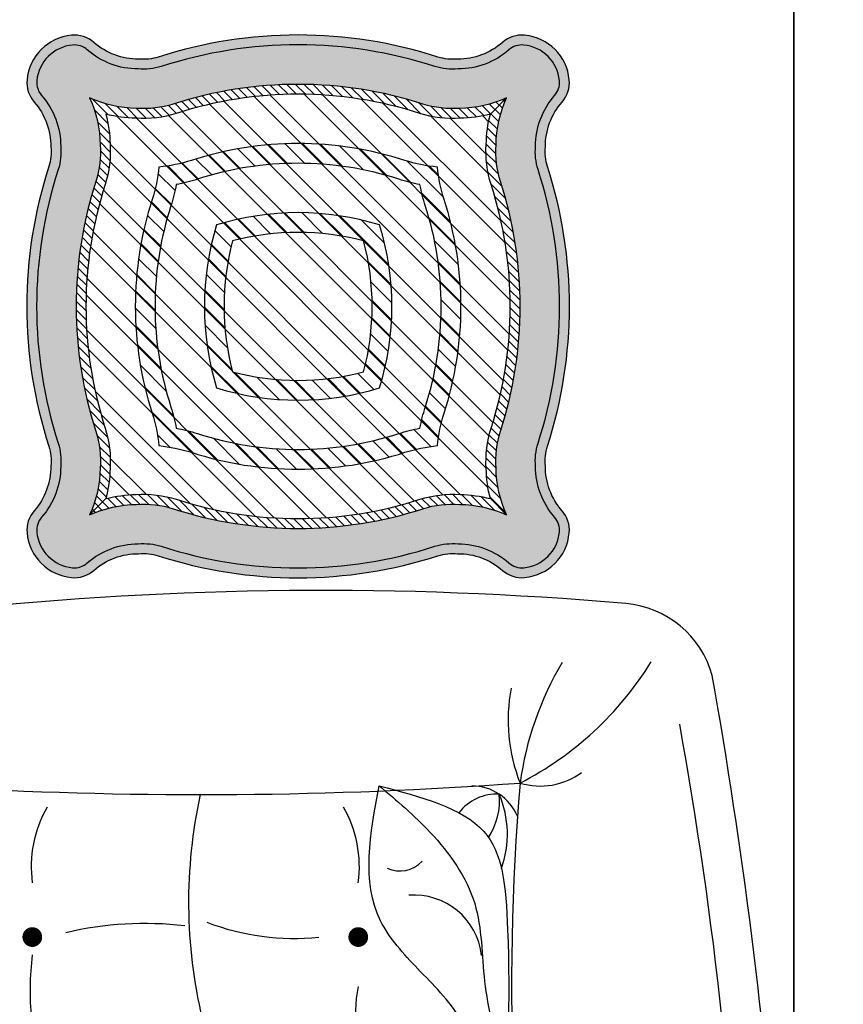
# Model space of a CAD drawing. Units: inches. Extents: x 844 to 2234, y 346 to 1084.
# Tile 88 of 93: x 2017.59 to 2030.9, y 712.93 to 728.83. Entities that reach past the tile are written whole.
import ezdxf

# ---------------------------------------------------------------- set-up
doc = ezdxf.new("R2010")
doc.units = ezdxf.units.IN
doc.header["$MEASUREMENT"] = 0
for name, color, linetype, lineweight in [('A-ANNO-DIMS', 2, 'Continuous', 18), ('A-WALL', 7, 'Continuous', 35), ('furniture', 8, 'Continuous', 18)]:
    doc.layers.add(name, color=color, linetype=linetype, lineweight=lineweight)
for name, color, linetype in [('RA-AP-01$0$FURN', 3, 'Continuous'), ('RA-AP-01$0$steel', 193, 'Continuous'), ('RA-AP-01$0$WOOD', 64, 'Continuous')]:
    doc.layers.add(name, color=color, linetype=linetype)
doc.styles.get("Standard").update_dxf_attribs({"font": 'arial.ttf'})
doc.dimstyles.get("Standard").update_dxf_attribs({"dimtxt": 6, "dimasz": 3, "dimexe": 0.18, "dimexo": 0.0625, "dimgap": 0.09, "dimtad": 0, "dimtih": 1, "dimtoh": 1, "dimdec": 1, "dimzin": 0, "dimdsep": 46, "dimlunit": 3, "dimtxsty": 'Standard', "dimblk": 'ARCHTICK', "dimcen": 0.09, "dimadec": 0, "dimazin": 0, "dimtfac": 1, "dimtdec": 1, "dimtofl": 0, "dimtmove": 0, "dimatfit": 3, "dimfxl": 1, "dimtolj": 1, "dimtzin": 0, "dimarcsym": 0})
pattern_1 = [(45, (0, 1.362436106329781), (-0.0088388347648318, 0.0088388347648318), [])]
pattern_2 = [(45, (0, 1.362436106329781), (-0.0044194173824159, 0.0044194173824159), [])]

# ---------------------------------------------------------------- blocks, each defined once
blk = doc.blocks.new('A$C2FCF5309')
at = {"layer": 'RA-AP-01$0$FURN'}
h = blk.add_hatch(dxfattribs=at)
h.set_pattern_fill('ANSI31', color=256, scale=0.1, style=0)
h.set_pattern_definition(pattern_1)
h.paths.add_polyline_path([(5.038683893313746, -5.169250834004607, -0.1583983521602212), (5.038683893312098, -5.373464580902012, 0.0306258898943267), (5.033304057242972, -5.394827569605182, 0.0306258898948892), (5.01194106853941, -5.40020740567441, -0.1028142994996694), (4.878286182323899, -5.414871334512708), (4.863600873530158, -5.43331743520547, 0.1120482678681049), (5.018059823131753, -5.419248541734471, -0.052642197802937), (5.050972078299936, -5.412495590662115, -0.0526421977994963), (5.057725029371615, -5.379583335496025, 0.1583028414702701), (5.057725029372958, -5.163132079409654, -0.052642197806903), (5.050972078299777, -5.130219824239078, -0.0526421977995126), (5.018059823133679, -5.123466873167369, 0.0215995840215353), (4.988903013548211, -5.115372132362452), (4.975007495303644, -5.132826183367946, -0.0289147572844802), (5.011941068537408, -5.142508009226167, 0.0306258898976746), (5.033304057242868, -5.147887845296027, 0.0306258899022411)])
h.paths.add_polyline_path([(4.975007495303645, -5.132826183367946), (4.988903013548211, -5.115372132362452, 0.1362374241599938), (4.801608567045604, -5.12346687316654, -0.0526421978036853), (4.768696311876971, -5.130219824239102, -0.05264219780204), (4.761943360804856, -5.163132079406747, 0.1583028414743723), (4.761943360806116, -5.379583335498449, -0.0526421977955461), (4.768696311877141, -5.412495590662114, -0.0526421978073986), (4.801608567048022, -5.419248541735437, 0.0454484293938888), (4.863600873530158, -5.43331743520547), (4.878286182323899, -5.414871334512708, -0.0546933379798044), (4.80772732164382, -5.40020740567649, 0.030625889903973), (4.786364332934043, -5.394827569605216, 0.0306258898932853), (4.780984496865101, -5.373464580902791, -0.1583983521638281), (4.780984496864308, -5.169250834000963, 0.03062588989692), (4.786364332933943, -5.147887845296004, 0.0306258898946324), (4.807727321637318, -5.142508009226805, -0.1288932573266927)])
h.paths.add_polyline_path([(4.843422214712861, -5.204945727074827, -0.0783685831716868), (4.924134454130224, -5.196727409635105), (4.939146578618322, -5.177870798323143, 0.1012675676854134), (4.827248748758957, -5.188772261120899, 0.1253648873081696), (4.820394258584192, -5.327034652050361), (4.837127701354095, -5.306015906404253, -0.0981593964869636)], flags=17)
h.paths.add_polyline_path([(4.843422214712824, -5.337769687826355, -0.0311091841722656), (4.837127701354095, -5.306015906404253), (4.820394258584193, -5.32703465205036, 0.0247727657431944), (4.827248748758908, -5.353943153780261, 0.0812754385032542), (4.916962478476905, -5.36629034358622), (4.933684093813825, -5.345286454285511, -0.0876255421014372)], flags=17)
h.paths.add_polyline_path([(4.992419641418037, -5.353943153780226, 0.1506053783834298), (4.992419641417933, -5.188772261120954, 0.0485966419124224), (4.939146578618321, -5.177870798323143), (4.924134454130224, -5.196727409635105, -0.0507799419579301), (4.976246175464031, -5.204945727074882, -0.1296645318906876), (4.97624617546411, -5.337769687826316, -0.0415667119298777), (4.933684093813825, -5.345286454285511), (4.916962478476905, -5.36629034358622, 0.0684915676023693)], flags=17)
h = blk.add_hatch(dxfattribs=at)
h.set_pattern_fill('ANSI31', color=256, scale=0.1, style=0)
h.set_pattern_definition(pattern_1)
h.paths.add_polyline_path([(5.038683893313746, -5.169250834004607, -0.1583983521602212), (5.038683893312098, -5.373464580902012, 0.0306258898943267), (5.033304057242972, -5.394827569605182, 0.0306258898948892), (5.01194106853941, -5.40020740567441, -0.1028142994996694), (4.878286182323899, -5.414871334512708), (4.863600873530158, -5.43331743520547, 0.1120482678681049), (5.018059823131753, -5.419248541734471, -0.052642197802937), (5.050972078299936, -5.412495590662115, -0.0526421977994963), (5.057725029371615, -5.379583335496025, 0.1583028414702701), (5.057725029372958, -5.163132079409654, -0.052642197806903), (5.050972078299777, -5.130219824239078, -0.0526421977995126), (5.018059823133679, -5.123466873167369, 0.0215995840215353), (4.988903013548211, -5.115372132362452), (4.975007495303644, -5.132826183367946, -0.0289147572844802), (5.011941068537408, -5.142508009226167, 0.0306258898976746), (5.033304057242868, -5.147887845296027, 0.0306258899022411)])
h.paths.add_polyline_path([(4.975007495303645, -5.132826183367946), (4.988903013548211, -5.115372132362452, 0.1362374241599938), (4.801608567045604, -5.12346687316654, -0.0526421978036853), (4.768696311876971, -5.130219824239102, -0.05264219780204), (4.761943360804856, -5.163132079406747, 0.1583028414743723), (4.761943360806116, -5.379583335498449, -0.0526421977955461), (4.768696311877141, -5.412495590662114, -0.0526421978073986), (4.801608567048022, -5.419248541735437, 0.0454484293938888), (4.863600873530158, -5.43331743520547), (4.878286182323899, -5.414871334512708, -0.0546933379798044), (4.80772732164382, -5.40020740567649, 0.030625889903973), (4.786364332934043, -5.394827569605216, 0.0306258898932853), (4.780984496865101, -5.373464580902791, -0.1583983521638281), (4.780984496864308, -5.169250834000963, 0.03062588989692), (4.786364332933943, -5.147887845296004, 0.0306258898946324), (4.807727321637318, -5.142508009226805, -0.1288932573266927)])
h.paths.add_polyline_path([(4.843422214712861, -5.204945727074827, -0.0783685831716868), (4.924134454130224, -5.196727409635105), (4.939146578618322, -5.177870798323143, 0.1012675676854134), (4.827248748758957, -5.188772261120899, 0.1253648873081696), (4.820394258584192, -5.327034652050361), (4.837127701354095, -5.306015906404253, -0.0981593964869636)], flags=17)
h.paths.add_polyline_path([(4.843422214712824, -5.337769687826355, -0.0311091841722656), (4.837127701354095, -5.306015906404253), (4.820394258584193, -5.32703465205036, 0.0247727657431944), (4.827248748758908, -5.353943153780261, 0.0812754385032542), (4.916962478476905, -5.36629034358622), (4.933684093813825, -5.345286454285511, -0.0876255421014372)], flags=17)
h.paths.add_polyline_path([(4.992419641418037, -5.353943153780226, 0.1506053783834298), (4.992419641417933, -5.188772261120954, 0.0485966419124224), (4.939146578618321, -5.177870798323143), (4.924134454130224, -5.196727409635105, -0.0507799419579301), (4.976246175464031, -5.204945727074882, -0.1296645318906876), (4.97624617546411, -5.337769687826316, -0.0415667119298777), (4.933684093813825, -5.345286454285511), (4.916962478476905, -5.36629034358622, 0.0684915676023693)], flags=17)
at = {"layer": 'RA-AP-01$0$WOOD'}
h = blk.add_hatch(color=256, dxfattribs=at)
edge = h.paths.add_edge_path()
edge.add_arc((4.683001772622394, -5.026441828662609), 0.0299999999999998, 48.77105092035535, 95.25687599427813)
edge.add_arc((4.684834195088484, -5.046357707450686), 0.0499999999998897, 95.25687599443106, 174.7431240064049)
edge.add_arc((4.664918316300367, -5.044525284985046), 0.0300000000000005, 174.7431240062535, 221.2289490796905)
edge.add_arc((4.591236830209155, -5.109094338216345), 0.0679700159630267, -0.5333070513215148, 41.228949079691915, ccw=False)
edge.add_arc((4.609451302807284, -5.114694777173187), 0.0500000000000008, -17.3556839752095, 5.7020707654044145, ccw=False)
edge.add_arc((5.095208119646659, -5.271357707450659), 0.4603971832811796, 162.0683908477609, 197.9316091523306)
edge.add_arc((4.609451302807533, -5.428020637728902), 0.0500000000000006, -5.702070765320514, 17.355683975293914, ccw=False)
edge.add_arc((4.591236830209412, -5.433621076685779), 0.0679700159630261, -41.228949079600625, 0.5333070514128053, ccw=False)
edge.add_arc((4.664918316300727, -5.498190129916959), 0.0299999999999995, 138.7710509204022, 185.256875994324)
edge.add_arc((4.684834195088642, -5.496357707450695), 0.0499999999997451, 185.2568759946742, 264.74312400432)
edge.add_arc((4.683001772622394, -5.516273586238612), 0.03, 264.743124003969, 311.2289490796446)
edge.add_arc((4.747570825853633, -5.589955072329876), 0.0679700159630271, 89.4666929486321, 131.2289490796457, ccw=False)
edge.add_arc((4.753171264810493, -5.57174059973175), 0.0500000000000015, 72.64431602474701, 95.70207076536133, ccw=False)
edge.add_arc((4.909834195088355, -5.085983782892503), 0.4603971832811774, 252.0683908477147, 287.9316091522845)
edge.add_arc((5.06649712536621, -5.57174059973175), 0.0499999999999999, 84.29792923463953, 107.35568397525361, ccw=False)
edge.add_arc((5.072097564323069, -5.589955072329877), 0.0679700159630274, 48.771050920354185, 90.5333070513679, ccw=False)
edge.add_arc((5.136666617554309, -5.516273586238614), 0.0299999999999997, 228.771050920353, 275.2568759942969)
edge.add_arc((5.134834195088338, -5.496357707450417), 0.0499999999999982, 275.2568759942949, 354.7431240057633)
edge.add_arc((5.154750073876535, -5.498190129916372), 0.0299999999999999, 354.7431240057662, 401.2289490796891)
edge.add_arc((5.228431559967749, -5.433621076685074), 0.0679700159630274, 179.4666929486771, 221.2289490796903, ccw=False)
edge.add_arc((5.210217087369615, -5.428020637728227), 0.0499999999999976, 162.6443160247947, 185.7020707654089, ccw=False)
edge.add_arc((4.724460270530244, -5.271357707450757), 0.4603971832811793, 342.0683908477607, 377.9316091523305)
edge.add_arc((5.210217087369368, -5.114694777172509), 0.0500000000000019, 174.2979292346878, 197.355683975302, ccw=False)
edge.add_arc((5.228431559967489, -5.109094338215639), 0.0679700159630279, 138.7710509203993, 180.5333070514128, ccw=False)
edge.add_arc((5.154750073876174, -5.044525284984457), 0.0300000000000001, 318.771050920401, 365.2568759954636)
edge.add_arc((5.13483419508816, -5.046357707450624), 0.0499999999998349, 5.256875995237118, 84.74312400549572)
edge.add_arc((5.136666617554308, -5.026441828662608), 0.0299999999999994, 84.74312400572185, 131.2289490796446)
edge.add_arc((5.072097564323072, -4.952760342571343), 0.0679700159630261, 269.4666929486298, 311.22894907964354, ccw=False)
edge.add_arc((5.066497125366206, -4.97097481516947), 0.0499999999999992, 252.64431602475162, 275.70207076536565, ccw=False)
edge.add_arc((4.909834195088355, -5.456731632008717), 0.4603971832811764, 72.06839084771546, 107.9316091522853)
edge.add_arc((4.753171264810493, -4.970974815169471), 0.0500000000000016, 264.2979292346387, 287.355683975253, ccw=False)
edge.add_arc((4.747570825853633, -4.952760342571346), 0.0679700159630274, 228.7710509203543, 270.5333070513679, ccw=False)
edge = h.paths.add_edge_path(flags=16)
edge.add_arc((4.683001772622395, -5.026441828662608), 0.019999999999999, 48.7710509203555, 95.2568759942793)
edge.add_arc((4.684834195088469, -5.046357707450671), 0.0399999999998731, 95.2568759944489, 174.7431240064248)
edge.add_arc((4.664918316300404, -5.044525284985035), 0.020000000000036, 174.7431240062186, 221.2289490796461)
edge.add_arc((4.591236830209151, -5.109094338216346), 0.0779700159630296, -0.13764630038667747, 41.228949079689585, ccw=False)
edge.add_arc((4.609451302807307, -5.11469477717304), 0.060000000000024, -17.406127045137907, 5.176192161068002, ccw=False)
edge.add_arc((5.09520811964665, -5.271357707450659), 0.4503971832811708, 162.0623235129628, 197.9376764869162)
edge.add_arc((4.609451302807532, -5.428020637728943), 0.0599999999999982, -5.176192160466428, 17.406127046715312, ccw=False)
edge.add_arc((4.591236830209414, -5.433621076685778), 0.0779700159630257, -41.2289490796029, 0.13764630095249686, ccw=False)
edge.add_arc((4.664918316300731, -5.498190129916961), 0.0200000000000047, 138.7710509204103, 185.2568759943212)
edge.add_arc((4.684834195088606, -5.496357707450731), 0.0399999999997066, 185.2568759947174, 264.7431240043665)
edge.add_arc((4.683001772622369, -5.516273586238541), 0.020000000000069, 264.7431240038842, 311.2289490795622)
edge.add_arc((4.747570825853635, -5.589955072329884), 0.0779700159630344, 89.8623536987642, 131.2289490796432, ccw=False)
edge.add_arc((4.753171264810603, -5.571740599731771), 0.0599999999999895, 72.5938729544394, 95.1761921602253, ccw=False)
edge.add_arc((4.909834195088365, -5.085983782892505), 0.4503971832811724, 252.0623235129989, 287.9376764870498)
edge.add_arc((5.066497125366216, -5.571740599731755), 0.0600000000000047, 84.8238078399923, 107.40612704528041, ccw=False)
edge.add_arc((5.072097564322998, -5.589955072329853), 0.077970015963056, 48.771050920303594, 90.13764630126451, ccw=False)
edge.add_arc((5.136666617554307, -5.516273586238622), 0.0199999999999931, 228.771050920344, 275.2568759943037)
edge.add_arc((5.134834195088338, -5.496357707450416), 0.0400000000000004, 275.2568759942928, 354.7431240057607)
edge.add_arc((5.154750073876533, -5.498190129916375), 0.0200000000000037, 354.7431240057783, 401.2289490796939)
edge.add_arc((5.228431559967745, -5.433621076685076), 0.0779700159630239, 179.8623536995147, 221.2289490796908, ccw=False)
edge.add_arc((5.210217087369586, -5.428020637728345), 0.0600000000000054, 162.5938729554486, 185.1761921609759, ccw=False)
edge.add_arc((4.724460270530243, -5.271357707450766), 0.4503971832811826, 342.0623235128896, 377.937676486982)
edge.add_arc((5.210217087369347, -5.114694777172486), 0.0599999999999777, 174.8238078387611, 197.4061270462219, ccw=False)
edge.add_arc((5.228431559967523, -5.109094338215542), 0.0779700159629885, 138.7710509204687, 180.1376463004423, ccw=False)
edge.add_arc((5.154750073876175, -5.044525284984459), 0.0199999999999989, 318.771050920406, 365.2568759954698)
edge.add_arc((5.134834195088138, -5.046357707450646), 0.0399999999998586, 5.256875995208452, 84.74312400546732)
edge.add_arc((5.136666617554292, -5.02644182866256), 0.0199999999999529, 84.74312400577769, 131.2289490797025)
edge.add_arc((5.072097564323069, -4.952760342571338), 0.077970015963032, 269.86235369901414, 311.2289490796421, ccw=False)
edge.add_arc((5.06649712536618, -4.97097481516946), 0.0600000000000007, 252.5938729548277, 275.17619216047467, ccw=False)
edge.add_arc((4.909834195088353, -5.456731632008716), 0.4503971832811739, 72.06232351293887, 107.9376764867365)
edge.add_arc((4.753171264810429, -4.970974815169467), 0.0599999999999991, 264.82380783985815, 287.40612704769893, ccw=False)
edge.add_arc((4.747570825853681, -4.952760342571361), 0.0779700159630467, 228.7710509203206, 270.13764630113724, ccw=False)
h = blk.add_hatch(color=256, dxfattribs=at)
edge = h.paths.add_edge_path()
edge.add_arc((4.683001772622395, -5.026441828662608), 0.019999999999999, 48.7710509203555, 95.2568759942793)
edge.add_arc((4.684834195088469, -5.046357707450671), 0.0399999999998731, 95.2568759944489, 174.7431240064248)
edge.add_arc((4.664918316300404, -5.044525284985035), 0.020000000000036, 174.7431240062186, 221.2289490796461)
edge.add_arc((4.591236830209151, -5.109094338216346), 0.0779700159630296, -0.13764630038667747, 41.228949079689585, ccw=False)
edge.add_arc((4.609451302807307, -5.11469477717304), 0.060000000000024, -17.406127045137907, 5.176192161068002, ccw=False)
edge.add_arc((5.09520811964665, -5.271357707450659), 0.4503971832811708, 162.0623235129628, 197.9376764869162)
edge.add_arc((4.609451302807532, -5.428020637728943), 0.0599999999999982, -5.176192160466428, 17.406127046715312, ccw=False)
edge.add_arc((4.591236830209414, -5.433621076685778), 0.0779700159630257, -41.2289490796029, 0.13764630095249686, ccw=False)
edge.add_arc((4.664918316300731, -5.498190129916961), 0.0200000000000047, 138.7710509204103, 185.2568759943212)
edge.add_arc((4.684834195088606, -5.496357707450731), 0.0399999999997066, 185.2568759947174, 264.7431240043665)
edge.add_arc((4.683001772622369, -5.516273586238541), 0.020000000000069, 264.7431240038842, 311.2289490795622)
edge.add_arc((4.747570825853635, -5.589955072329884), 0.0779700159630344, 89.8623536987642, 131.2289490796432, ccw=False)
edge.add_arc((4.753171264810603, -5.571740599731771), 0.0599999999999895, 72.5938729544394, 95.1761921602253, ccw=False)
edge.add_arc((4.909834195088365, -5.085983782892505), 0.4503971832811724, 252.0623235129989, 287.9376764870498)
edge.add_arc((5.066497125366216, -5.571740599731755), 0.0600000000000047, 84.8238078399923, 107.40612704528041, ccw=False)
edge.add_arc((5.072097564322998, -5.589955072329853), 0.077970015963056, 48.771050920303594, 90.13764630126451, ccw=False)
edge.add_arc((5.136666617554307, -5.516273586238622), 0.0199999999999931, 228.771050920344, 275.2568759943037)
edge.add_arc((5.134834195088338, -5.496357707450416), 0.0400000000000004, 275.2568759942928, 354.7431240057607)
edge.add_arc((5.154750073876533, -5.498190129916375), 0.0200000000000037, 354.7431240057783, 401.2289490796939)
edge.add_arc((5.228431559967745, -5.433621076685076), 0.0779700159630239, 179.8623536995147, 221.2289490796908, ccw=False)
edge.add_arc((5.210217087369586, -5.428020637728345), 0.0600000000000054, 162.5938729554486, 185.1761921609759, ccw=False)
edge.add_arc((4.724460270530243, -5.271357707450766), 0.4503971832811826, 342.0623235128896, 377.937676486982)
edge.add_arc((5.210217087369347, -5.114694777172486), 0.0599999999999777, 174.8238078387611, 197.4061270462219, ccw=False)
edge.add_arc((5.228431559967523, -5.109094338215542), 0.0779700159629885, 138.7710509204687, 180.1376463004423, ccw=False)
edge.add_arc((5.154750073876175, -5.044525284984459), 0.0199999999999989, 318.771050920406, 365.2568759954698)
edge.add_arc((5.134834195088138, -5.046357707450646), 0.0399999999998586, 5.256875995208452, 84.74312400546732)
edge.add_arc((5.136666617554292, -5.02644182866256), 0.0199999999999529, 84.74312400577769, 131.2289490797025)
edge.add_arc((5.072097564323069, -4.952760342571338), 0.077970015963032, 269.86235369901414, 311.2289490796421, ccw=False)
edge.add_arc((5.06649712536618, -4.97097481516946), 0.0600000000000007, 252.5938729548277, 275.17619216047467, ccw=False)
edge.add_arc((4.909834195088353, -5.456731632008716), 0.4503971832811739, 72.06232351293887, 107.9376764867365)
edge.add_arc((4.753171264810429, -4.970974815169467), 0.0599999999999991, 264.82380783985815, 287.40612704769893, ccw=False)
edge.add_arc((4.747570825853681, -4.952760342571361), 0.0779700159630467, 228.7710509203206, 270.13764630113724, ccw=False)
edge = h.paths.add_edge_path(flags=16)
edge.add_arc((4.591236830209151, -5.109094338216348), 0.1179700159630308, 0.7417751874182841, 24.563326950263672, ccw=False)
edge.add_arc((4.609451302807302, -5.114694777173093), 0.100000000000012, -17.52836504564658, 4.087328884225087, ccw=False)
edge.add_arc((5.095208119646651, -5.271357707450657), 0.4103971832811724, 162.0403002448777, 197.9596997550675)
edge.add_arc((4.60945130280753, -5.428020637728918), 0.1000000000000027, -4.087328883827581, 17.528365046291924, ccw=False)
edge.add_arc((4.591236830209414, -5.433621076685779), 0.1179700159630246, 335.43667305041845, 359.2582248129738, ccw=False)
edge.add_arc((4.747570825853596, -5.589955072329891), 0.117970015963042, 90.7417751868461, 114.5633269496104, ccw=False)
edge.add_arc((4.753171264810559, -5.571740599731767), 0.0999999999999976, 72.47163495370341, 94.0873288836737, ccw=False)
edge.add_arc((4.909834195088367, -5.085983782892503), 0.4103971832811735, 252.0403002449999, 287.9596997551833)
edge.add_arc((5.066497125366205, -5.571740599731755), 0.1000000000000057, 85.91267111645209, 107.5283650455624, ccw=False)
edge.add_arc((5.072097564322985, -5.58995507232986), 0.117970015963046, 65.4366730497672, 89.25822481317113, ccw=False)
edge.add_arc((5.22843155996773, -5.433621076684992), 0.1179700159630096, 180.7417751873964, 204.5633269502712, ccw=False)
edge.add_arc((5.210217087369591, -5.428020637728301), 0.0999999999999969, 162.4716349546276, 184.0873288841682, ccw=False)
edge.add_arc((4.724460270530243, -5.271357707450766), 0.4103971832811825, 342.0403002448147, 377.9596997550345)
edge.add_arc((5.210217087369347, -5.114694777172489), 0.0999999999999796, 175.9126711156995, 197.5283650464392, ccw=False)
edge.add_arc((5.228431559967512, -5.109094338215525), 0.1179700159630019, 155.4366730502992, 179.2582248126247, ccw=False)
edge.add_arc((5.072097564323172, -4.952760342571314), 0.1179700159630537, 270.74177518697286, 294.56332694975765, ccw=False)
edge.add_arc((5.066497125366189, -4.970974815169462), 0.1000000000000017, 252.471634954247, 274.0873288838353, ccw=False)
edge.add_arc((4.909834195088353, -5.456731632008716), 0.4103971832811758, 72.04030024486342, 107.9596997549354)
edge.add_arc((4.75317126481046, -4.970974815169467), 0.1000000000000041, 265.91267111635307, 287.5283650466103, ccw=False)
edge.add_arc((4.747570825853629, -4.952760342571342), 0.1179700159630538, 245.43667304992562, 269.2582248131125, ccw=False)
h = blk.add_hatch(dxfattribs=at)
h.set_pattern_fill('ANSI31', color=256, scale=0.05, style=0)
h.set_pattern_definition(pattern_2)
h.paths.add_polyline_path([(5.105336294329346, -5.394854099602528, 0.0940138826956367), (5.100476366643778, -5.435568764288975, 0.0606271852326483), (5.104678567100611, -5.466202079462671, 0.0606271852344644), (5.074045251925975, -5.46199987900586, 0.0940138827021426), (5.033330587236848, -5.466859806692645, -0.1305325492494615), (4.828072633169377, -5.477944178050054), (4.821119726105699, -5.486677669841435, 0.1336226599878005), (5.036379334063467, -5.476383803188216, -0.0945969211935747), (5.073624810952389, -5.471994942692536, -0.1043170707892296), (5.121137550891356, -5.48266106325342, -0.1043170707868944), (5.110471430330457, -5.435148323315565, -0.0945969211952573), (5.114860290825935, -5.397902846425963, 0.1580239521433527), (5.114860290826324, -5.144812568476775, -0.0945969212010491), (5.110471430330247, -5.10756709158498, -0.1043170707844371), (5.121137550890657, -5.060054351648168, -0.104317070786514), (5.073624810952866, -5.070720472208642, -0.0945969211958523), (5.036379334063063, -5.066331611712874, 0.1580239521426795), (4.783289056114906, -5.066331611712465, -0.0945969211985319), (4.746043579224103, -5.070720472208672, -0.1043170707882665), (4.698530839285552, -5.060054351647925, -0.1043170707867205), (4.709196959846443, -5.10756709158571, -0.094596921196788), (4.704808099350826, -5.144812568475902, 0.1580239521433127), (4.704808099350699, -5.397902846425022, -0.094596921197841), (4.709196959846712, -5.435148323315576, -0.1043170707855109), (4.698530839286393, -5.482661063252921, -0.1043170707864168), (4.746043579224162, -5.471994942692571, -0.0945969211977586), (4.783289056114671, -5.476383803188671, 0.0238966994662183), (4.821119726105699, -5.486677669841435), (4.828072633169378, -5.477944178050054, -0.0269814195959459), (4.786337802940177, -5.466859806692736, 0.0940138827039629), (4.745623138250268, -5.461999879005895, 0.0606271852320776), (4.714989823076826, -5.466202079462476, 0.0606271852304618), (4.719192023533341, -5.435568764289856, 0.0940138826917763), (4.714332095848404, -5.394854099604977, -0.1580706864542086), (4.714332095846561, -5.147861315302034, 0.0940138827032017), (4.719192023533127, -5.107146650612438, 0.0606271852329446), (4.714989823076289, -5.076513335438588, 0.0606271852340035), (4.745623138250698, -5.08071553589536, 0.0940138827025969), (4.786337802940015, -5.075855608208526, -0.1580706864508517), (5.033330587237968, -5.075855608208939, 0.0940138827009578), (5.074045251926627, -5.080715535895319, 0.0606271852322557), (5.104678567100159, -5.076513335438697, 0.0606271852308743), (5.100476366643561, -5.107146650611519, 0.0940138827178109), (5.105336294331983, -5.147861315307182, -0.1580706864490946)])
h = blk.add_hatch(dxfattribs=at)
h.set_pattern_fill('ANSI31', color=256, scale=0.05, style=0)
h.set_pattern_definition(pattern_2)
h.paths.add_polyline_path([(5.105336294329346, -5.394854099602528, 0.0940138826956367), (5.100476366643778, -5.435568764288975, 0.0606271852326483), (5.104678567100611, -5.466202079462671, 0.0606271852344644), (5.074045251925975, -5.46199987900586, 0.0940138827021426), (5.033330587236848, -5.466859806692645, -0.1305325492494615), (4.828072633169377, -5.477944178050054), (4.821119726105699, -5.486677669841435, 0.1336226599878005), (5.036379334063467, -5.476383803188216, -0.0945969211935747), (5.073624810952389, -5.471994942692536, -0.1043170707892296), (5.121137550891356, -5.48266106325342, -0.1043170707868944), (5.110471430330457, -5.435148323315565, -0.0945969211952573), (5.114860290825935, -5.397902846425963, 0.1580239521433527), (5.114860290826324, -5.144812568476775, -0.0945969212010491), (5.110471430330247, -5.10756709158498, -0.1043170707844371), (5.121137550890657, -5.060054351648168, -0.104317070786514), (5.073624810952866, -5.070720472208642, -0.0945969211958523), (5.036379334063063, -5.066331611712874, 0.1580239521426795), (4.783289056114906, -5.066331611712465, -0.0945969211985319), (4.746043579224103, -5.070720472208672, -0.1043170707882665), (4.698530839285552, -5.060054351647925, -0.1043170707867205), (4.709196959846443, -5.10756709158571, -0.094596921196788), (4.704808099350826, -5.144812568475902, 0.1580239521433127), (4.704808099350699, -5.397902846425022, -0.094596921197841), (4.709196959846712, -5.435148323315576, -0.1043170707855109), (4.698530839286393, -5.482661063252921, -0.1043170707864168), (4.746043579224162, -5.471994942692571, -0.0945969211977586), (4.783289056114671, -5.476383803188671, 0.0238966994662183), (4.821119726105699, -5.486677669841435), (4.828072633169378, -5.477944178050054, -0.0269814195959459), (4.786337802940177, -5.466859806692736, 0.0940138827039629), (4.745623138250268, -5.461999879005895, 0.0606271852320776), (4.714989823076826, -5.466202079462476, 0.0606271852304618), (4.719192023533341, -5.435568764289856, 0.0940138826917763), (4.714332095848404, -5.394854099604977, -0.1580706864542086), (4.714332095846561, -5.147861315302034, 0.0940138827032017), (4.719192023533127, -5.107146650612438, 0.0606271852329446), (4.714989823076289, -5.076513335438588, 0.0606271852340035), (4.745623138250698, -5.08071553589536, 0.0940138827025969), (4.786337802940015, -5.075855608208526, -0.1580706864508517), (5.033330587237968, -5.075855608208939, 0.0940138827009578), (5.074045251926627, -5.080715535895319, 0.0606271852322557), (5.104678567100159, -5.076513335438697, 0.0606271852308743), (5.100476366643561, -5.107146650611519, 0.0940138827178109), (5.105336294331983, -5.147861315307182, -0.1580706864490946)])
h = blk.add_hatch(dxfattribs=at)
h.set_pattern_fill('ANSI32,_I', color=256, scale=0.1, style=2)
h.set_pattern_definition([(45, (0, 0), (-0.0265165042944955, 0.0265165042944955), []), (45, (0.0176776695, 0), (-0.0265165042944955, 0.0265165042944955), [])])
h.paths.add_polyline_path([(4.843422214712824, -5.337769687826354, 0.1296645318905289), (4.97624617546411, -5.337769687826316, 0.1296645318906876), (4.976246175464032, -5.204945727074882, 0.129664531890418), (4.843422214712861, -5.204945727074827, 0.129664531890765)], flags=0)
h.paths.add_polyline_path([(5.039131224122924, -5.170637849998464, -0.0326520429852175), (5.033304057242868, -5.147887845296027, -0.0326520429894721), (5.010554052537512, -5.142060678415043, 0.1561383235202698), (4.809114337641437, -5.142060678414318, -0.0326520429925972), (4.786364332933944, -5.147887845296004, -0.0326520429914489), (4.780537166052582, -5.170637850002729, 0.1561383235189577), (4.780537166052134, -5.37207756489719, -0.0326520429934175), (4.786364332934042, -5.394827569605215, -0.0326520429823496), (4.809114337634529, -5.400654736484653, 0.156138323524066), (5.010554052535268, -5.400654736486903, -0.032652042992888), (5.033304057242972, -5.394827569605183, -0.0326520429928733), (5.039131224124712, -5.372077564897496, 0.1561383235226786)], flags=0)
h.paths.add_polyline_path([(4.992419641418037, -5.353943153780226, -0.1506053783832862), (4.827248748758909, -5.353943153780261, -0.1506053783835069), (4.827248748758957, -5.188772261120899, -0.1506053783831346), (4.992419641417933, -5.188772261120954, -0.1506053783834298)], flags=0)
h.paths.add_polyline_path([(4.976246175464111, -5.337769687826316, -0.1296645318905298), (4.843422214712824, -5.337769687826354, -0.129664531890765), (4.843422214712862, -5.204945727074827, -0.1296645318904162), (4.976246175464031, -5.204945727074882, -0.1296645318906876)], flags=0)
h.paths.add_polyline_path([(5.105721254232479, -5.149054940982025, -0.0968902512052664), (5.100476366643561, -5.107146650611519, -0.0606271852308743), (5.104678567100159, -5.076513335438697, -0.0606271852322574), (5.074045251926626, -5.080715535895319, -0.0968902512197216), (5.032136961550132, -5.075470648304253, 0.1564657949319774), (4.787531428625239, -5.075470648304682, -0.0968902512150626), (4.745623138250699, -5.08071553589536, -0.060627185234009), (4.714989823076288, -5.076513335438587, -0.0606271852329501), (4.719192023533127, -5.10714665061244, -0.0968902512185585), (4.713947135942331, -5.149054940988458, 0.1564657949285579), (4.713947135940853, -5.393660473908259, -0.0968902512319826), (4.71919202353334, -5.435568764289873, -0.0606271852304288), (4.714989823076825, -5.466202079462476, -0.0606271852320811), (4.745623138250269, -5.461999879005895, -0.0968902512162649), (4.787531428625332, -5.467244766596559, 0.1564657949327057), (5.032136961551311, -5.46724476659659, -0.0968902512153659), (5.074045251925975, -5.46199987900586, -0.0606271852344627), (5.10467856710061, -5.466202079462671, -0.0606271852326483), (5.100476366643777, -5.435568764288975, -0.0968902512258216), (5.105721254235559, -5.393660473909953, 0.1564657949340142)])
h.paths.add_polyline_path([(5.057725029371625, -5.379583335495999, 0.0526421977995391), (5.050972078299936, -5.412495590662114, 0.0526421978029782), (5.018059823131728, -5.419248541734479, -0.1583028414681072), (4.801608567048168, -5.419248541735485, 0.0526421978076402), (4.76869631187714, -5.412495590662113, 0.0526421977956189), (4.761943360806101, -5.379583335498404, -0.1583028414743129), (4.761943360804846, -5.163132079406778, 0.0526421978020944), (4.768696311876972, -5.130219824239101, 0.0526421978033651), (4.80160856704541, -5.123466873166602, -0.1583028414716875), (5.018059823133628, -5.123466873167353, 0.0526421977995944), (5.050972078299776, -5.130219824239078, 0.0526421978070423), (5.057725029372986, -5.163132079409739, -0.1583028414701848)], flags=16)
h.paths.add_polyline_path([(5.038683893312112, -5.373464580901968, 0.0306258898943915), (5.033304057242972, -5.394827569605182, 0.0306258898948892), (5.01194106853941, -5.40020740567441, -0.1583983521587032), (4.807727321643864, -5.400207405676503, 0.0306258899040366), (4.786364332934043, -5.394827569605215, 0.0306258898931986), (4.780984496865119, -5.37346458090285, -0.1583983521638542), (4.7809844968643, -5.169250834000989, 0.0306258898969596), (4.786364332933945, -5.147887845296004, 0.0306258898946195), (4.807727321637311, -5.142508009226808, -0.1583983521623412), (5.011941068537318, -5.142508009226139, 0.030625889897807), (5.033304057242868, -5.147887845296028, 0.0306258899020632), (5.038683893313706, -5.169250834004486, -0.1583983521602835)], flags=0)
for p, q in [((4.714989823076289, -5.076513335438588), (4.698530839285552, -5.060054351647925)), ((4.714989823076289, -5.076513335438588), (4.698530839285552, -5.060054351647925)), ((5.104678567100159, -5.076513335438697), (5.121137550890656, -5.060054351648169)), ((5.104678567100159, -5.076513335438697), (5.121137550890656, -5.060054351648169)), ((5.10467856710061, -5.466202079462671), (5.121137550891355, -5.482661063253419)), ((5.10467856710061, -5.466202079462671), (5.121137550891355, -5.482661063253419))]:
    blk.add_line(p, q, dxfattribs=at)
for points in [[(4.702773858784635, -5.003879368495489, 0.2056608120285223), (4.680253138923443, -4.996568010480312, 0.3614336704708569), (4.635044498118043, -5.041776651286372, 0.2056608120263112), (4.642355856133262, -5.064297371147306, -0.1842662638101064), (4.65920390179375, -5.10972699154053, -0.1009492694051416), (4.657174869772992, -5.129609908955028, 0.1577727036674954), (4.657174869773219, -5.41310550594699, -0.1009492694051416), (4.659203901794006, -5.432988423361486, -0.1842662638101064), (4.64235585613359, -5.478418043754737, 0.2056608120285221), (4.635044498118431, -5.500938763615934, 0.3614336704593693), (4.680253138922529, -5.546147404420826, 0.2056608120364936), (4.702773858784635, -5.538836046405732, -0.1842662638101064), (4.748203479177874, -5.52198800074528, -0.1009492694051415), (4.768086396592371, -5.524017032766053, 0.1577727036674954), (5.051581993584332, -5.524017032766055, -0.1009492694051416), (5.071464910998829, -5.521988000745282, -0.1842662638101064), (5.116894531392067, -5.538836046405734, 0.2056608120286145), (5.13941525125327, -5.546147404420911, 0.3614336704683636), (5.184623892058835, -5.500938763615299, 0.2056608120285223), (5.177312534043641, -5.478418043754112, -0.1842662638101063), (5.160464488383153, -5.432988423360887, -0.1009492694051416), (5.162493520403909, -5.41310550594639, 0.1577727036674954), (5.162493520403684, -5.129609908954428, -0.1009492694051416), (5.160464488382894, -5.109726991539933, -0.1842662638101064), (5.17731253404331, -5.064297371146681, 0.2056608120337072), (5.184623892058415, -5.041776651284888, 0.3614336704623863), (5.139415251253259, -4.99656801048031, 0.2056608120285223), (5.116894531392067, -5.003879368495487, -0.1842662638101064), (5.071464910998829, -5.020727414155937, -0.1009492694051416), (5.051581993584332, -5.018698382135166, 0.1577727036674956), (4.768086396592371, -5.018698382135168, -0.1009492694051416), (4.748203479177874, -5.020727414155941, -0.1842662638101064)], [(4.702773858784635, -5.003879368495489, 0.2056608120285223), (4.680253138923443, -4.996568010480312, 0.3614336704708569), (4.635044498118043, -5.041776651286372, 0.2056608120263112), (4.642355856133262, -5.064297371147306, -0.1842662638101064), (4.65920390179375, -5.10972699154053, -0.1009492694051416), (4.657174869772992, -5.129609908955028, 0.1577727036674954), (4.657174869773219, -5.41310550594699, -0.1009492694051416), (4.659203901794006, -5.432988423361486, -0.1842662638101064), (4.64235585613359, -5.478418043754737, 0.2056608120285221), (4.635044498118431, -5.500938763615934, 0.3614336704593693), (4.680253138922529, -5.546147404420826, 0.2056608120364936), (4.702773858784635, -5.538836046405732, -0.1842662638101064), (4.748203479177874, -5.52198800074528, -0.1009492694051415), (4.768086396592371, -5.524017032766053, 0.1577727036674954), (5.051581993584332, -5.524017032766055, -0.1009492694051416), (5.071464910998829, -5.521988000745282, -0.1842662638101064), (5.116894531392067, -5.538836046405734, 0.2056608120286145), (5.13941525125327, -5.546147404420911, 0.3614336704683636), (5.184623892058835, -5.500938763615299, 0.2056608120285223), (5.177312534043641, -5.478418043754112, -0.1842662638101063), (5.160464488383153, -5.432988423360887, -0.1009492694051416), (5.162493520403909, -5.41310550594639, 0.1577727036674954), (5.162493520403684, -5.129609908954428, -0.1009492694051416), (5.160464488382894, -5.109726991539933, -0.1842662638101064), (5.17731253404331, -5.064297371146681, 0.2056608120337072), (5.184623892058415, -5.041776651284888, 0.3614336704623863), (5.139415251253259, -4.99656801048031, 0.2056608120285223), (5.116894531392067, -5.003879368495487, -0.1842662638101064), (5.071464910998829, -5.020727414155937, -0.1009492694051416), (5.051581993584332, -5.018698382135166, 0.1577727036674956), (4.768086396592371, -5.018698382135168, -0.1009492694051416), (4.748203479177874, -5.020727414155941, -0.1842662638101064)], [(4.696183163397222, -5.011400188551196, 0.2056608120285295), (4.681169350156427, -5.006525949874411, 0.3614336704708588), (4.645002437512154, -5.042692862519237, 0.2056608120262659), (4.649876676188964, -5.057706675759887, -0.182481815856965), (4.669206621172843, -5.109281651732388, -0.0988540857970112), (4.666703803477437, -5.13264334722805, 0.1578269695851905), (4.666703803477144, -5.410072067672365, -0.0988540858013112), (4.6692066211731, -5.433433763168966, -0.1824818158591246), (4.649876676189301, -5.485008739142145, 0.2056608120284717), (4.64500243751253, -5.500022552382944, 0.3614336704593821), (4.681169350155757, -5.536189465026749, 0.2056608120365057), (4.696183163397221, -5.531315226350026, -0.1824818158605826), (4.747758139370833, -5.51198528136619, -0.0988540857951607), (4.771119834866025, -5.514488099061806, 0.1578269695856264), (5.04854855531107, -5.514488099061688, -0.0988540857929677), (5.071910250805761, -5.511985281366138, -0.1824818158609529), (5.123485226779481, -5.531315226350027, 0.2056608120286893), (5.138499040020282, -5.536189465026812, 0.3614336704683556), (5.174665952664737, -5.500022552382323, 0.2056608120284882), (5.169791713987938, -5.485008739141532, -0.1824818158574124), (5.150461769004059, -5.4334337631689, -0.0988540857940221), (5.152964586699289, -5.410072067673927, 0.1578269695858123), (5.1529645866996, -5.132643347228565, -0.0988540858025403), (5.150461769003872, -5.109281651731659, -0.1824818158565006), (5.169791713987599, -5.057706675759273, 0.2056608120337192), (5.174665952664335, -5.042692862518078, 0.3614336704623903), (5.138499040020236, -5.006525949874406, 0.2056608120285323), (5.123485226779481, -5.011400188551195, -0.1824818158594503), (5.071910250806212, -5.03073013353503, -0.09885408579455), (5.048548555311143, -5.028227315839558, 0.1578269695844942), (4.771119834867991, -5.028227315838772, -0.0988540858042156), (4.747758139370745, -5.030730133535067, -0.1824818158603032)], [(4.696183163397222, -5.011400188551196, 0.2056608120285295), (4.681169350156427, -5.006525949874411, 0.3614336704708588), (4.645002437512154, -5.042692862519237, 0.2056608120262659), (4.649876676188964, -5.057706675759887, -0.182481815856965), (4.669206621172843, -5.109281651732388, -0.0988540857970112), (4.666703803477437, -5.13264334722805, 0.1578269695851905), (4.666703803477144, -5.410072067672365, -0.0988540858013112), (4.6692066211731, -5.433433763168966, -0.1824818158591246), (4.649876676189301, -5.485008739142145, 0.2056608120284717), (4.64500243751253, -5.500022552382944, 0.3614336704593821), (4.681169350155757, -5.536189465026749, 0.2056608120365057), (4.696183163397221, -5.531315226350026, -0.1824818158605826), (4.747758139370833, -5.51198528136619, -0.0988540857951607), (4.771119834866025, -5.514488099061806, 0.1578269695856264), (5.04854855531107, -5.514488099061688, -0.0988540857929677), (5.071910250805761, -5.511985281366138, -0.1824818158609529), (5.123485226779481, -5.531315226350027, 0.2056608120286893), (5.138499040020282, -5.536189465026812, 0.3614336704683556), (5.174665952664737, -5.500022552382323, 0.2056608120284882), (5.169791713987938, -5.485008739141532, -0.1824818158574124), (5.150461769004059, -5.4334337631689, -0.0988540857940221), (5.152964586699289, -5.410072067673927, 0.1578269695858123), (5.1529645866996, -5.132643347228565, -0.0988540858025403), (5.150461769003872, -5.109281651731659, -0.1824818158565006), (5.169791713987599, -5.057706675759273, 0.2056608120337192), (5.174665952664335, -5.042692862518078, 0.3614336704623903), (5.138499040020236, -5.006525949874406, 0.2056608120285323), (5.123485226779481, -5.011400188551195, -0.1824818158594503), (5.071910250806212, -5.03073013353503, -0.09885408579455), (5.048548555311143, -5.028227315839558, 0.1578269695844942), (4.771119834867991, -5.028227315838772, -0.0988540858042156), (4.747758139370745, -5.030730133535067, -0.1824818158603032)], [(4.698530839285552, -5.060054351647925, -0.1043170707867612), (4.709196959846444, -5.107567091585729, -0.0945969211969405), (4.704808099350802, -5.144812568475978, 0.1580239521432241), (4.704808099350681, -5.397902846424963, -0.0945969211980322), (4.709196959846711, -5.43514832331559, -0.104317070785482), (4.698530839286393, -5.482661063252921, -0.1043170707864036), (4.746043579224155, -5.471994942692571, -0.094596921197375), (4.78328905611452, -5.476383803188623, 0.1580239521431959), (5.036379334063463, -5.476383803188218, -0.0945969211935888), (5.07362481095239, -5.471994942692536, -0.1043170707892253), (5.121137550891355, -5.482661063253419, -0.1043170707868921), (5.110471430330457, -5.435148323315565, -0.0945969211954828), (5.114860290825962, -5.397902846425878, 0.158023952143358), (5.114860290826295, -5.144812568476682, -0.0945969212007617), (5.110471430330247, -5.107567091584995, -0.1043170707844689), (5.121137550890656, -5.060054351648169, -0.1043170707864946), (5.073624810952874, -5.070720472208642, -0.0945969211956941), (5.036379334063131, -5.066331611712896, 0.1580239521426976), (4.783289056114946, -5.066331611712452, -0.0945969211986379), (4.746043579224103, -5.070720472208672, -0.1043170707882684)], [(4.698530839285552, -5.060054351647925, -0.1043170707867612), (4.709196959846444, -5.107567091585729, -0.0945969211969405), (4.704808099350802, -5.144812568475978, 0.1580239521432241), (4.704808099350681, -5.397902846424963, -0.0945969211980322), (4.709196959846711, -5.43514832331559, -0.104317070785482), (4.698530839286393, -5.482661063252921, -0.1043170707864036), (4.746043579224155, -5.471994942692571, -0.094596921197375), (4.78328905611452, -5.476383803188623, 0.1580239521431959), (5.036379334063463, -5.476383803188218, -0.0945969211935888), (5.07362481095239, -5.471994942692536, -0.1043170707892253), (5.121137550891355, -5.482661063253419, -0.1043170707868921), (5.110471430330457, -5.435148323315565, -0.0945969211954828), (5.114860290825962, -5.397902846425878, 0.158023952143358), (5.114860290826295, -5.144812568476682, -0.0945969212007617), (5.110471430330247, -5.107567091584995, -0.1043170707844689), (5.121137550890656, -5.060054351648169, -0.1043170707864946), (5.073624810952874, -5.070720472208642, -0.0945969211956941), (5.036379334063131, -5.066331611712896, 0.1580239521426976), (4.783289056114946, -5.066331611712452, -0.0945969211986379), (4.746043579224103, -5.070720472208672, -0.1043170707882684)], [(4.714989823076289, -5.076513335438588, -0.0606271852329464), (4.719192023533127, -5.107146650612439, -0.0940138827030756), (4.714332095846578, -5.147861315301983, 0.1580706864542707), (4.714332095848417, -5.394854099605018, -0.0940138826916965), (4.719192023533341, -5.435568764289864, -0.0606271852304462), (4.714989823076826, -5.466202079462476, -0.0606271852320585), (4.745623138250258, -5.461999879005895, -0.0940138827037036), (4.786337802940059, -5.466859806692699, 0.1580706864500221), (5.033330587236783, -5.466859806692666, -0.0940138827023111), (5.074045251925979, -5.46199987900586, -0.060627185234454), (5.10467856710061, -5.466202079462671, -0.0606271852326709), (5.100476366643777, -5.435568764288963, -0.0940138826958686), (5.105336294329379, -5.394854099602421, 0.1580706864489859), (5.105336294331999, -5.147861315307237, -0.0940138827179432), (5.100476366643561, -5.107146650611518, -0.0606271852308726), (5.104678567100159, -5.076513335438697, -0.0606271852322592), (5.074045251926625, -5.080715535895319, -0.094013882701022), (5.03333058723794, -5.075855608208931, 0.1580706864508015), (4.786337802940061, -5.075855608208511, -0.0940138827027143), (4.745623138250695, -5.08071553589536, -0.0606271852339983)], [(4.714989823076289, -5.076513335438588, -0.0606271852329464), (4.719192023533127, -5.107146650612439, -0.0940138827030756), (4.714332095846578, -5.147861315301983, 0.1580706864542707), (4.714332095848417, -5.394854099605018, -0.0940138826916965), (4.719192023533341, -5.435568764289864, -0.0606271852304462), (4.714989823076826, -5.466202079462476, -0.0606271852320585), (4.745623138250258, -5.461999879005895, -0.0940138827037036), (4.786337802940059, -5.466859806692699, 0.1580706864500221), (5.033330587236783, -5.466859806692666, -0.0940138827023111), (5.074045251925979, -5.46199987900586, -0.060627185234454), (5.10467856710061, -5.466202079462671, -0.0606271852326709), (5.100476366643777, -5.435568764288963, -0.0940138826958686), (5.105336294329379, -5.394854099602421, 0.1580706864489859), (5.105336294331999, -5.147861315307237, -0.0940138827179432), (5.100476366643561, -5.107146650611518, -0.0606271852308726), (5.104678567100159, -5.076513335438697, -0.0606271852322592), (5.074045251926625, -5.080715535895319, -0.094013882701022), (5.03333058723794, -5.075855608208931, 0.1580706864508015), (4.786337802940061, -5.075855608208511, -0.0940138827027143), (4.745623138250695, -5.08071553589536, -0.0606271852339983)], [(4.768696311876972, -5.130219824239102, -0.0526421978019087), (4.761943360804882, -5.163132079406667, 0.1583028414744761), (4.761943360806133, -5.379583335498504, -0.0526421977954539), (4.76869631187714, -5.412495590662113, -0.0526421978076619), (4.801608567048181, -5.419248541735488, 0.1583028414681522), (5.0180598231318, -5.419248541734456, -0.0526421978028585), (5.050972078299936, -5.412495590662114, -0.0526421977992923), (5.057725029371576, -5.379583335496149, 0.1583028414703719), (5.057725029372956, -5.163132079409646, -0.0526421978068888), (5.050972078299776, -5.130219824239078, -0.052642197799403), (5.018059823133745, -5.12346687316739, 0.1583028414717216), (4.801608567045482, -5.123466873166579, -0.0526421978034837)], [(4.768696311876972, -5.130219824239102, -0.0526421978019087), (4.761943360804882, -5.163132079406667, 0.1583028414744761), (4.761943360806133, -5.379583335498504, -0.0526421977954539), (4.76869631187714, -5.412495590662113, -0.0526421978076619), (4.801608567048181, -5.419248541735488, 0.1583028414681522), (5.0180598231318, -5.419248541734456, -0.0526421978028585), (5.050972078299936, -5.412495590662114, -0.0526421977992923), (5.057725029371576, -5.379583335496149, 0.1583028414703719), (5.057725029372956, -5.163132079409646, -0.0526421978068888), (5.050972078299776, -5.130219824239078, -0.052642197799403), (5.018059823133745, -5.12346687316739, 0.1583028414717216), (4.801608567045482, -5.123466873166579, -0.0526421978034837)], [(4.786364332933944, -5.147887845296004, -0.0306258898969254), (4.780984496864308, -5.169250834000966, 0.1583983521638412), (4.780984496865107, -5.373464580902811, -0.0306258898932568), (4.786364332934043, -5.394827569605216, -0.0306258899041339), (4.80772732164393, -5.400207405676526, 0.1583983521586416), (5.011941068539401, -5.400207405674413, -0.0306258898949021), (5.033304057242972, -5.394827569605182, -0.0306258898943513), (5.038683893312104, -5.373464580901996, 0.1583983521602784), (5.038683893313717, -5.16925083400452, -0.0306258899021139), (5.033304057242868, -5.147887845296027, -0.030625889897777), (5.011941068537338, -5.142508009226145, 0.1583983521624288), (4.807727321637224, -5.142508009226835, -0.0306258898944937)], [(4.786364332933944, -5.147887845296004, -0.0306258898969254), (4.780984496864308, -5.169250834000966, 0.1583983521638412), (4.780984496865107, -5.373464580902811, -0.0306258898932568), (4.786364332934043, -5.394827569605216, -0.0306258899041339), (4.80772732164393, -5.400207405676526, 0.1583983521586416), (5.011941068539401, -5.400207405674413, -0.0306258898949021), (5.033304057242972, -5.394827569605182, -0.0306258898943513), (5.038683893312104, -5.373464580901996, 0.1583983521602784), (5.038683893313717, -5.16925083400452, -0.0306258899021139), (5.033304057242868, -5.147887845296027, -0.030625889897777), (5.011941068537338, -5.142508009226145, 0.1583983521624288), (4.807727321637224, -5.142508009226835, -0.0306258898944937)], [(4.827248748758957, -5.1887722611209, 0.1506053783835061), (4.827248748758908, -5.353943153780261, 0.150605378383287), (4.992419641418037, -5.353943153780226, 0.1506053783834298), (4.992419641417933, -5.188772261120954, 0.1506053783831346)], [(4.827248748758957, -5.1887722611209, 0.1506053783835061), (4.827248748758908, -5.353943153780261, 0.150605378383287), (4.992419641418037, -5.353943153780226, 0.1506053783834298), (4.992419641417933, -5.188772261120954, 0.1506053783831346)], [(4.843422214712861, -5.204945727074827, 0.1296645318907659), (4.843422214712824, -5.337769687826355, 0.1296645318905299), (4.976246175464111, -5.337769687826316, 0.1296645318906876), (4.976246175464032, -5.204945727074882, 0.129664531890418)], [(4.843422214712861, -5.204945727074827, 0.1296645318907659), (4.843422214712824, -5.337769687826355, 0.1296645318905299), (4.976246175464111, -5.337769687826316, 0.1296645318906876), (4.976246175464032, -5.204945727074882, 0.129664531890418)]]:
    blk.add_lwpolyline(points, format="xyb", close=True, dxfattribs=at)
blk = doc.blocks.new('A$C7EE91E48')
at = {"layer": 'RA-AP-01$0$FURN', "const_width": 0.01}
for points in [[(9.624035873781274, -9.001865189332936, 1), (9.624035873781297, -8.991865189332932, 1)], [(9.624035873780826, -9.322250169057511, -1), (9.624035873780826, -9.332250169057513, -1)]]:
    blk.add_lwpolyline(points, format="xyb", close=True, dxfattribs=at)
at = {"layer": 'RA-AP-01$0$FURN'}
for centre, radius, start, end in [((14.24233490628227, -9.167687782925107), 4.473931917517753, 176.7828902523826, 184.1477233631118), ((6.42249118116022, -9.291612252417751), 3.552808610866049, 355.0473312316413, 6.058872375658039), ((9.56961973833057, -9.296929112294796), 0.3023568492824586, 83.09448255116675, 107.588060785551), ((9.695285873781074, -9.11718462924615), 0.1214118203512435, 60.14190744855965, 97.69166328915595), ((9.286001211781066, -9.111007490545871), 0.3517162425384579, 353.4124896676112, 13.16745705655713), ((9.65905457432348, -9.665283690153952), 0.5100538472773755, 77.61824893593078, 103.3122231353938), ((9.866927508269418, -9.261753835450415), 0.2442261434243043, 158.9017070735605, 185.9923925191661), ((9.695285873780948, -9.206930729144496), 0.1214118203512435, 262.3083367106845, 299.8580925512809), ((9.547087767231618, -9.453923781794167), 0.1295083186917369, 77.99013392028127, 121.3796151021958), ((9.721962050880482, -9.369186052387374), 0.0310151388417235, 155.7760318513891, 227.3789451550393), ((9.597674721851437, -9.383696092249494), 0.0689028341546707, 276.4195171090914, 4.461572645688697), ((9.721016980434092, -9.467332461384675), 0.0478550828899777, 356.575295631534, 52.68338292382147), ((9.727193091302688, -9.442442658911482), 0.05, 292.5826724246039, 359.9999999990535), ((9.76257267867739, -9.40215366480788), 0.0683206773889159, 236.6729861493448, 275.2183950426369), ((9.728288059321612, -9.374174170762846), 0.1042084262671507, 250.4828318717156, 292.8692939327817), ((9.57476488929157, -11.93482586084473), 2.452160434589619, 85.19614643967464, 99.84577117055878), ((9.843355501572116, -9.648968385188004), 0.1698955038956699, 78.87784313594504, 111.8512383801196), ((9.847560443890684, -9.511725524783945), 0.0704710051510922, 163.1338634205325, 216.4126496157095), ((9.736702898899553, -9.812515797398348), 0.3241573581843151, 59.29856748426889, 82.3026350986056), ((10.0808517727553, -9.33652322886128), 0.3382138395168437, 207.2303327094028, 238.2563708342648), ((9.862408234899569, -9.589702786759155), 0.1, 285.499494600857, 355.0473312316416), ((9.079565375949262, -5.436149540861864), 4.284827979137255, 272.1916353285572, 280.2199257473579), ((8.936022170067632, -4.284064429245874), 5.485438776325237, 268.8504034693488, 280.0060732220913)]:
    blk.add_arc(centre, radius, start, end, dxfattribs=at)
for points, knots in [([(9.777267912908336, -9.348473919394923), (9.72881227229245, -9.339303204541801), (9.658611784301481, -9.326017059735285), (9.588175161652856, -9.390102169424527), (9.54880260620782, -9.431527358661508), (9.430932710956684, -9.481194893850247), (9.632509618052595, -9.481144249541359), (9.745531325142556, -9.470177725074079), (9.766284889927373, -9.39059173320999), (9.777267912908336, -9.348473919394923)], [0, 0, 0, 0, 0.1367586589314793, 0.1981301758052369, 0.2677729570689282, 0.3281194902553322, 0.4737578340741565, 0.5765194025309516, 0.692033228742226, 0.692033228742226, 0.692033228742226, 0.692033228742226]), ([(9.777267912908336, -9.348473919394923), (9.762308671078125, -9.366257458082648), (9.729176734078989, -9.405644687068653), (9.66202804490802, -9.45323209587751), (9.577043610038041, -9.451871670355906), (9.52447597485284, -9.465284086012414), (9.497548572726195, -9.472154501784399)], [0, 0, 0, 0, 0.0700185406710175, 0.1550780383534523, 0.2344491945777067, 0.3178048737568313, 0.3178048737568313, 0.3178048737568313, 0.3178048737568313])]:
    blk.add_open_spline(points, degree=3, knots=knots, dxfattribs=at)
blk = doc.blocks.new('A$C5D2F253E')
at = {"layer": 'RA-AP-01$0$steel', "xscale": -1}
blk.add_blockref('A$C2FCF5309', (6.339960502260055, 7.248884637679282), dxfattribs=at)
at = {"layer": 'RA-AP-01$0$WOOD', "xscale": -1, "rotation": 180}
blk.add_blockref('A$C7EE91E48', (-8.833013809079146, -7.288751725733902), dxfattribs=at)
blk = doc.blocks.new('_ArchTick')
at = {"color": 0, "linetype": 'ByBlock', "const_width": 0.15}
blk.add_lwpolyline([(-0.5, -0.5), (0.5, 0.5)], dxfattribs=at)
blk = doc.blocks.new('*D121')
at = {"layer": 'A-ANNO-DIMS', "color": 0, "lineweight": -2, "transparency": 16777216}
for p, q in [((2030.271987351997, 734.262611118704), (2040.245275089302, 734.262611118704)), ((2040.065275089302, 734.262611118704), (2040.065275089302, 704.6043509484256)), ((2040.065275089302, 668.557359536674), (2040.065275089302, 698.2156197069523)), ((2030.271987351997, 668.557359536674), (2040.245275089302, 668.557359536674))]:
    blk.add_line(p, q, dxfattribs=at)
at = {"layer": 'Defpoints', "color": 0, "transparency": 16777216}
for p in [(2030.209487351997, 734.262611118704), (2040.065275089302, 734.262611118704), (2030.209487351997, 668.557359536674)]:
    blk.add_point(p, dxfattribs=at)
at = {"layer": 'A-ANNO-DIMS', "color": 0, "lineweight": -2, "transparency": 16777216, "xscale": 3, "yscale": 3, "zscale": 3}
for p, rotation in [((2040.065275089302, 734.262611118704), 90), ((2040.065275089302, 668.557359536674), 270)]:
    blk.add_blockref('_ArchTick', p, dxfattribs=dict(at, rotation=rotation))
at = {"layer": 'A-ANNO-DIMS', "color": 0, "transparency": 16777216, "insert": (2040.065275089302, 701.4099853276883), "char_height": 6, "attachment_point": 5}
blk.add_mtext('\\A1;LOUNGE SET 5\'-5 1/2" TYP.', dxfattribs=at)

msp = doc.modelspace()

# ---------------------------------------------------------------- linework, layer by layer
at = {"layer": 'A-WALL'}
msp.add_line((2030.099168352677, 766.4551697629895), (2030.099168352677, 629.4551697629895), dxfattribs=at)

# ---------------------------------------------------------------- block references
at = {"layer": 'furniture', "xscale": -15.94108302203742, "yscale": 15.94108302203742, "zscale": 15.94108302203742, "rotation": 270}
msp.add_blockref('A$C5D2F253E', (1990.567271852805, 701.4028671565849), dxfattribs=at)

# ---------------------------------------------------------------- dimensions: what is measured, and where the dimension line sits
at = {"layer": 'A-ANNO-DIMS'}
dim = msp.add_linear_dim(base=(2040.065275089302, 734.262611118704), p1=(2030.209487351996, 668.5573595366737), p2=(2030.209487351996, 734.2626111187037), angle=90, text='LOUNGE SET <> TYP.', dimstyle='Standard', override={"dimdec": 1, "dimlfac": 1, "dimrnd": 0, "dimzin": 1, "dimdsep": 46, "dimlunit": 4, "dimfrac": 2}, dxfattribs=at)
dim.commit()
dim.dimension.update_dxf_attribs({"geometry": '*D121', "text_midpoint": (2040.065275089302, 701.4099853276883)})

doc.saveas('drawing.dxf')
